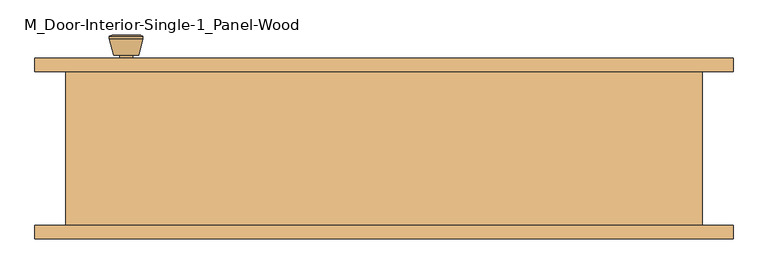
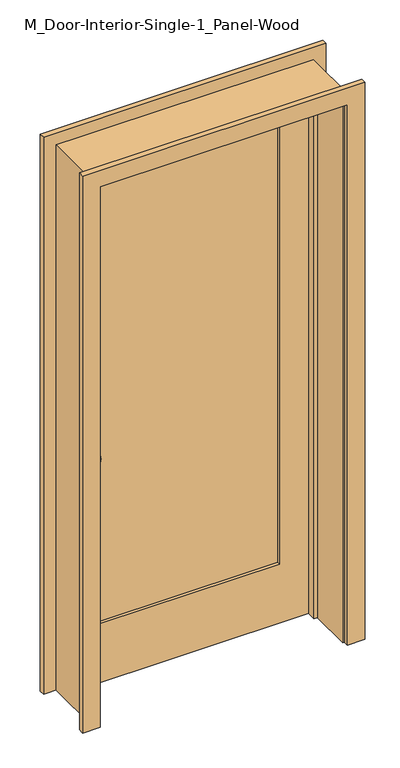
"""IFC4 building model written with IfcOpenShell, lengths in millimetres: door geometry, M_Door-Interior-Single-1_Panel-Wood."""

from ifc_helpers import new_model, si_unit, point, frame, frame_2d, origin, place, context, project, spatial, polyline, circle_curve, trimmed, segment, composite_curve, outline, extrude, faceted_brep, source, transform, mapped, element, save
from ifc_brep_helpers import plane_surface, cylinder_surface, revolved_surface, advanced_brep


def m_door_interior_single_1_panel_wood_d38da9c5(model_context):
    return source(origin(), model_context, "Body", "SolidModel", [
        advanced_brep(
        [(-385.0, 70.825, 914.4), (-375.0, 70.825, 914.4), (-395.0, 70.825, 914.4), (-364.5241324, 21.825, 914.4), (-385.0, 21.825, 914.4), (-405.4758676, 21.825, 914.4), (-360.0, 23.6528681, 914.4), (-410.0, 23.6528681, 914.4), (-360.0, 27.1165463, 914.4), (-410.0, 27.1165463, 914.4), (-366.363764, 51.825, 914.4), (-403.636236, 51.825, 914.4), (-375.0, 51.825, 914.4), (-395.0, 51.825, 914.4)],
        [
            (0, 1),
            (1, 2, circle_curve(frame((-385.0, 70.825, 914.4), z_axis=(0.0, 1.0, 0.0), x_axis=(-1.0, 0.0, 0.0)), 10.0)),
            (2, 0),
            (2, 1, circle_curve(frame((-385.0, 70.825, 914.4), z_axis=(0.0, 1.0, 0.0), x_axis=(-1.0, 0.0, 0.0)), 10.0)),
            (3, 4),
            (4, 5),
            (5, 3, circle_curve(frame((-385.0, 21.825, 914.4), z_axis=(0.0, -1.0, 0.0), x_axis=(-1.0, 0.0, 0.0)), 20.4758676)),
            (3, 5, circle_curve(frame((-385.0, 21.825, 914.4), z_axis=(0.0, -1.0, 0.0), x_axis=(-1.0, 0.0, 0.0)), 20.4758676)),
            (6, 3),
            (5, 7),
            (7, 6, circle_curve(frame((-385.0, 23.6528681, 914.4), z_axis=(0.0, -1.0, 0.0), x_axis=(-1.0, 0.0, 0.0)), 25.0)),
            (6, 7, circle_curve(frame((-385.0, 23.6528681, 914.4), z_axis=(0.0, -1.0, 0.0), x_axis=(-1.0, 0.0, 0.0)), 25.0)),
            (8, 6),
            (7, 9),
            (9, 8, circle_curve(frame((-385.0, 27.1165463, 914.4), z_axis=(0.0, -1.0, 0.0), x_axis=(-1.0, 0.0, 0.0)), 25.0)),
            (8, 9, circle_curve(frame((-385.0, 27.1165463, 914.4), z_axis=(0.0, -1.0, 0.0), x_axis=(-1.0, 0.0, 0.0)), 25.0)),
            (10, 8),
            (9, 11),
            (11, 10, circle_curve(frame((-385.0, 51.825, 914.4), z_axis=(0.0, -1.0, 0.0), x_axis=(-1.0, 0.0, 0.0)), 18.636236)),
            (10, 11, circle_curve(frame((-385.0, 51.825, 914.4), z_axis=(0.0, -1.0, 0.0), x_axis=(-1.0, 0.0, 0.0)), 18.636236)),
            (12, 10),
            (11, 13),
            (13, 12, circle_curve(frame((-385.0, 51.825, 914.4), z_axis=(0.0, -1.0, 0.0), x_axis=(-1.0, 0.0, 0.0)), 10.0)),
            (12, 13, circle_curve(frame((-385.0, 51.825, 914.4), z_axis=(0.0, -1.0, 0.0), x_axis=(-1.0, 0.0, 0.0)), 10.0)),
            (1, 12),
            (13, 2),
        ],
        [
            plane_surface(frame((-385.0, 70.825, 914.4), z_axis=(0.0, 1.0, 0.0), x_axis=(-1.0, 0.0, 0.0))),
            plane_surface(frame((-385.0, 21.825, 914.4), z_axis=(0.0, -1.0, 0.0), x_axis=(-1.0, 0.0, 0.0))),
            revolved_surface(polyline([(-405.4758676, 21.825, 914.4), (-410.0, 23.6528681, 914.4)]), (-385.0, 70.825, 914.4), (0.0, 1.0, 0.0)),
            cylinder_surface(frame((-385.0, 70.825, 914.4), z_axis=(0.0, 1.0, 0.0), x_axis=(-1.0, 0.0, 0.0)), 25.0),
            revolved_surface(polyline([(-410.0, 27.1165463, 914.4), (-403.636236, 51.825, 914.4)]), (-385.0, 70.825, 914.4), (0.0, 1.0, 0.0)),
            plane_surface(frame((-385.0, 51.825, 914.4), z_axis=(0.0, 1.0, 0.0), x_axis=(-1.0, 0.0, 0.0))),
            cylinder_surface(frame((-385.0, 70.825, 914.4), z_axis=(0.0, 1.0, 0.0), x_axis=(-1.0, 0.0, 0.0)), 10.0),
        ],
        [
            (0, [[1, 2, 3]]),
            (0, [[-3, 4, -1]]),
            (1, [[5, 6, 7]]),
            (1, [[-6, -5, 8]]),
            (2, [[9, -7, 10, 11]]),
            (2, [[-10, -8, -9, 12]]),
            (3, [[13, -11, 14, 15]]),
            (3, [[-14, -12, -13, 16]]),
            (4, [[17, -15, 18, 19]]),
            (4, [[-18, -16, -17, 20]]),
            (5, [[21, -19, 22, 23]]),
            (5, [[-22, -20, -21, 24]]),
            (6, [[25, -23, 26, -2]]),
            (6, [[-26, -24, -25, -4]]),
        ],
    ),
        extrude(outline(composite_curve([segment(trimmed(circle_curve(frame_2d((914.4, -385.0)), 30.0), [point((914.4, -415.0))], [point((914.4, -355.0))], False, "CARTESIAN"), True, "CONTINUOUS"), segment(trimmed(circle_curve(frame_2d((914.4, -385.0)), 30.0), [point((914.4, -355.0))], [point((914.4, -415.0))], False, "CARTESIAN"), True, "CONTINUOUS")], self_intersect=False)), frame((0.0, 70.825, 0.0), z_axis=(0.0, 1.0, 0.0), x_axis=(0.0, 0.0, 1.0)), (0.0, 0.0, 1.0), 6.0),
        advanced_brep(
        [(-385.0, 117.825, 914.4), (-395.0, 117.825, 914.4), (-375.0, 117.825, 914.4), (-364.5241324, 166.825, 914.4), (-405.4758676, 166.825, 914.4), (-385.0, 166.825, 914.4), (-360.0, 164.9971319, 914.4), (-410.0, 164.9971319, 914.4), (-360.0, 161.5334537, 914.4), (-410.0, 161.5334537, 914.4), (-366.363764, 136.825, 914.4), (-403.636236, 136.825, 914.4), (-375.0, 136.825, 914.4), (-395.0, 136.825, 914.4)],
        [
            (0, 1),
            (1, 2, circle_curve(frame((-385.0, 117.825, 914.4), z_axis=(0.0, -1.0, 0.0), x_axis=(-1.0, 0.0, 0.0)), 10.0)),
            (2, 0),
            (2, 1, circle_curve(frame((-385.0, 117.825, 914.4), z_axis=(0.0, -1.0, 0.0), x_axis=(-1.0, 0.0, 0.0)), 10.0)),
            (3, 4, circle_curve(frame((-385.0, 166.825, 914.4), z_axis=(0.0, 1.0, 0.0), x_axis=(-1.0, 0.0, 0.0)), 20.4758676)),
            (4, 5),
            (5, 3),
            (4, 3, circle_curve(frame((-385.0, 166.825, 914.4), z_axis=(0.0, 1.0, 0.0), x_axis=(-1.0, 0.0, 0.0)), 20.4758676)),
            (6, 7, circle_curve(frame((-385.0, 164.9971319, 914.4), z_axis=(0.0, 1.0, 0.0), x_axis=(-1.0, 0.0, 0.0)), 25.0)),
            (7, 4),
            (3, 6),
            (7, 6, circle_curve(frame((-385.0, 164.9971319, 914.4), z_axis=(0.0, 1.0, 0.0), x_axis=(-1.0, 0.0, 0.0)), 25.0)),
            (8, 9, circle_curve(frame((-385.0, 161.5334537, 914.4), z_axis=(0.0, 1.0, 0.0), x_axis=(-1.0, 0.0, 0.0)), 25.0)),
            (9, 7),
            (6, 8),
            (9, 8, circle_curve(frame((-385.0, 161.5334537, 914.4), z_axis=(0.0, 1.0, 0.0), x_axis=(-1.0, 0.0, 0.0)), 25.0)),
            (10, 11, circle_curve(frame((-385.0, 136.825, 914.4), z_axis=(0.0, 1.0, 0.0), x_axis=(-1.0, 0.0, 0.0)), 18.636236)),
            (11, 9),
            (8, 10),
            (11, 10, circle_curve(frame((-385.0, 136.825, 914.4), z_axis=(0.0, 1.0, 0.0), x_axis=(-1.0, 0.0, 0.0)), 18.636236)),
            (12, 13, circle_curve(frame((-385.0, 136.825, 914.4), z_axis=(0.0, 1.0, 0.0), x_axis=(-1.0, 0.0, 0.0)), 10.0)),
            (13, 11),
            (10, 12),
            (13, 12, circle_curve(frame((-385.0, 136.825, 914.4), z_axis=(0.0, 1.0, 0.0), x_axis=(-1.0, 0.0, 0.0)), 10.0)),
            (1, 13),
            (12, 2),
        ],
        [
            plane_surface(frame((-385.0, 117.825, 914.4), z_axis=(0.0, -1.0, 0.0), x_axis=(-1.0, 0.0, 0.0))),
            plane_surface(frame((-385.0, 166.825, 914.4), z_axis=(0.0, 1.0, 0.0), x_axis=(-1.0, 0.0, 0.0))),
            revolved_surface(polyline([(-405.4758676, 166.825, 914.4), (-410.0, 164.9971319, 914.4)]), (-385.0, 117.825, 914.4), (0.0, -1.0, 0.0)),
            cylinder_surface(frame((-385.0, 117.825, 914.4), z_axis=(0.0, -1.0, 0.0), x_axis=(-1.0, 0.0, 0.0)), 25.0),
            revolved_surface(polyline([(-410.0, 161.5334537, 914.4), (-403.636236, 136.825, 914.4)]), (-385.0, 117.825, 914.4), (0.0, -1.0, 0.0)),
            plane_surface(frame((-385.0, 136.825, 914.4), z_axis=(0.0, -1.0, 0.0), x_axis=(-1.0, 0.0, 0.0))),
            cylinder_surface(frame((-385.0, 117.825, 914.4), z_axis=(0.0, -1.0, 0.0), x_axis=(-1.0, 0.0, 0.0)), 10.0),
        ],
        [
            (0, [[1, 2, 3]]),
            (0, [[-3, 4, -1]]),
            (1, [[5, 6, 7]]),
            (1, [[8, -7, -6]]),
            (2, [[9, 10, -5, 11]]),
            (2, [[12, -11, -8, -10]]),
            (3, [[13, 14, -9, 15]]),
            (3, [[16, -15, -12, -14]]),
            (4, [[17, 18, -13, 19]]),
            (4, [[20, -19, -16, -18]]),
            (5, [[21, 22, -17, 23]]),
            (5, [[24, -23, -20, -22]]),
            (6, [[-2, 25, -21, 26]]),
            (6, [[-4, -26, -24, -25]]),
        ],
    ),
        extrude(outline(composite_curve([segment(trimmed(circle_curve(frame_2d((914.4, -385.0)), 30.0), [point((914.4, -415.0))], [point((914.4, -355.0))], False, "CARTESIAN"), True, "CONTINUOUS"), segment(trimmed(circle_curve(frame_2d((914.4, -385.0)), 30.0), [point((914.4, -355.0))], [point((914.4, -415.0))], False, "CARTESIAN"), True, "CONTINUOUS")], self_intersect=False)), frame((0.0, 111.825, 0.0), z_axis=(0.0, 1.0, 0.0), x_axis=(0.0, 0.0, 1.0)), (0.0, 0.0, 1.0), 6.0),
        faceted_brep([(475.0, 111.825, 0.0), (475.0, -118.175, 0.0), (450.0, -118.175, 0.0), (450.0, 41.9, 0.0), (437.3, 41.9, 0.0), (437.3, 76.825, 0.0), (450.0, 76.825, 0.0), (450.0, 111.825, 0.0), (475.0, 111.825, 2125.0), (475.0, -118.175, 2125.0), (-475.0, -118.175, 2125.0), (-475.0, -118.175, 0.0), (-450.0, -118.175, 0.0), (-450.0, -118.175, 2100.0), (450.0, -118.175, 2100.0), (450.0, 41.9, 2100.0), (-450.0, 41.9, 2100.0), (-450.0, 41.9, 0.0), (-437.3, 41.9, 0.0), (-437.3, 41.9, 2087.3), (437.3, 41.9, 2087.3), (437.3, 76.825, 2087.3), (-437.3, 76.825, 2087.3), (-437.3, 76.825, 0.0), (-450.0, 76.825, 0.0), (-450.0, 76.825, 2100.0), (450.0, 76.825, 2100.0), (450.0, 111.825, 2100.0), (-450.0, 111.825, 2100.0), (-450.0, 111.825, 0.0), (-475.0, 111.825, 0.0), (-475.0, 111.825, 2125.0)], [[[0, 1, 2, 3, 4, 5, 6, 7]], [[1, 0, 8, 9]], [[2, 1, 9, 10, 11, 12, 13, 14]], [[3, 2, 14, 15]], [[4, 3, 15, 16, 17, 18, 19, 20]], [[5, 4, 20, 21]], [[6, 5, 21, 22, 23, 24, 25, 26]], [[7, 6, 26, 27]], [[0, 7, 27, 28, 29, 30, 31, 8]], [[9, 8, 31, 10]], [[15, 14, 13, 16]], [[21, 20, 19, 22]], [[27, 26, 25, 28]], [[30, 29, 24, 23, 18, 17, 12, 11]], [[10, 31, 30, 11]], [[16, 13, 12, 17]], [[22, 19, 18, 23]], [[28, 25, 24, 29]]]),
        extrude(outline(polyline([(2100.0, -450.0), (0.0, -450.0), (0.0, 450.0), (2100.0, 450.0), (2100.0, -450.0)]), holes=[polyline([(1980.0, -330.0), (1980.0, 330.0), (230.0, 330.0), (230.0, -330.0), (1980.0, -330.0)])]), frame((0.0, 76.825, 0.0), z_axis=(0.0, 1.0, 0.0), x_axis=(0.0, 0.0, 1.0)), (0.0, 0.0, 1.0), 35.0),
        extrude(outline(polyline([(330.0, 88.4916667), (-330.0, 88.4916667), (-330.0, 100.1583333), (330.0, 100.1583333), (330.0, 88.4916667)])), frame((0.0, 0.0, 230.0), z_axis=(0.0, 0.0, 1.0), x_axis=(1.0, 0.0, 0.0)), (0.0, 0.0, 1.0), 1750.0),
        extrude(outline(polyline([(0.0, 456.35), (0.0, 521.35), (2171.35, 521.35), (2171.35, -521.35), (0.0, -521.35), (0.0, -456.35), (2106.35, -456.35), (2106.35, 456.35), (0.0, 456.35)])), frame((0.0, 111.825, 0.0), z_axis=(0.0, 1.0, 0.0), x_axis=(0.0, 0.0, 1.0)), (0.0, 0.0, 1.0), 20.0),
        extrude(outline(polyline([(0.0, 456.35), (0.0, 521.35), (2171.35, 521.35), (2171.35, -521.35), (0.0, -521.35), (0.0, -456.35), (2106.35, -456.35), (2106.35, 456.35), (0.0, 456.35)])), frame((0.0, -138.175, 0.0), z_axis=(0.0, 1.0, 0.0), x_axis=(0.0, 0.0, 1.0)), (0.0, 0.0, 1.0), 20.0),
    ])


if __name__ == "__main__":
    model = new_model("IFC4")
    model_context = context("Model", 3, world=origin())
    ifc_project = project(units=[si_unit("LENGTHUNIT", "METRE", prefix="MILLI")], contexts=[model_context])
    site = spatial("IfcSite", under=ifc_project)
    building = spatial("IfcBuilding", under=site)
    placement = place(None, origin())
    m_door_interior_single_1_panel_wood_shape = m_door_interior_single_1_panel_wood_d38da9c5(model_context)
    element("IfcDoor", 1, ObjectType="M_Door-Interior-Single-1_Panel-Wood", at=placement, inside=building, context=model_context, shape_type="MappedRepresentation", body=[
        mapped(m_door_interior_single_1_panel_wood_shape, transform((0.0, 0.0, 0.0), x_axis=(1.0, 0.0, 0.0), y_axis=(0.0, 1.0, 0.0), z_axis=(0.0, 0.0, 1.0))),
    ])
    save(model, "model.ifc")

# Revit data of these elements
# Type "M_Door-Interior-Single-1_Panel-Wood"
#   Type Mark = "26"
#   Assembly Code = "C1020300"
#   Analytic Construction = "Wooden"
#   Top Rail = 120 mm
#   Thickness = 35 mm
#   Thermal Resistance (R) = 0.455703 (m²·K)/W
#   Swing Angle [instance default] = 90.00°
#   Stiles = 120 mm
#   Rough Width = 950 mm
#   Rough Height = 2125 mm
#   Height = 2100 mm
#   Width = 900 mm
#   Heat Transfer Coefficient (U) = 2.19465 W/(m²·K)
#   Bottom Rail = 230 mm
#   Trim Material = Cherry
#   Panel Material = Cherry
#   Frame Material = Cherry
#   Door Handle Material = Aluminum
#   Visual Light Transmittance = 0
#   Solar Heat Gain Coefficient = 0
#   Wall Closure = (empty or 0)
#   Function = (empty or 0)
# Element 1 (IfcDoor, "M_Door-Interior-Single-1_Panel-Wood")
#   Materials on its faces: "Cherry", "Aluminum"
# Materials
#   "Cherry": class "Wood", colour RGB 154 107 61, transparency 0, Description = "Prunus Serotina", Cost = 0
#   "Aluminum": class "Metal", colour RGB 244 244 244, transparency 0, Description = "Aluminum 6061", Cost = 0
